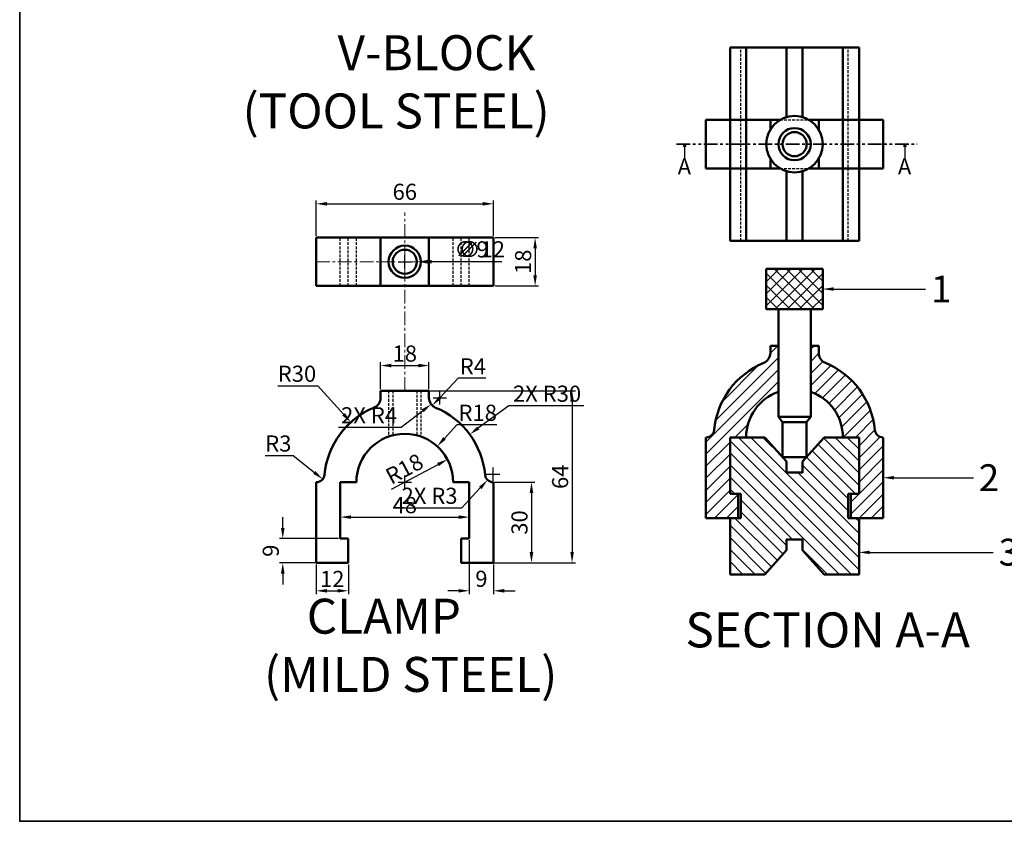
# Model space of a CAD drawing. Units: millimetres. Extents: x 0 to 624, y -214 to 340.
# Tile 1 of 3: x 0 to 366, y -214 to 84. Entities that reach past the tile are written whole.
import ezdxf
from ezdxf import colors
from ezdxf.entities.mleader import LeaderData, LeaderLine
from ezdxf.math import Vec2, Vec3

# ---------------------------------------------------------------- set-up
doc = ezdxf.new("R2010")
doc.units = ezdxf.units.MM
doc.header["$LTSCALE"] = 0.4
for name, pattern in [('CENTER', [50.8, 31.75, -6.35, 6.35, -6.35]), ('HIDDEN', [9.525, 6.35, -3.175]), ('PHANTOM', [63.5, 31.75, -6.35, 6.35, -6.35, 6.35, -6.35])]:
    doc.linetypes.add(name, pattern=pattern)
for name, color, linetype, lineweight in [('M-ANNO-SYMB', 6, 'Continuous', 25), ('M-CNTR', 1, 'CENTER', 18), ('M-DIMS', 2, 'Continuous', 25), ('M-HATC', 8, 'Continuous', 18), ('M-HIDN', 4, 'HIDDEN', 25), ('M-OUTL', 7, 'Continuous', 50), ('M-SECT', 6, 'PHANTOM', 35), ('M-TEXT', 3, 'Continuous', 25), ('M-TTLB', 7, 'Continuous', 35)]:
    doc.layers.add(name, color=color, linetype=linetype, lineweight=lineweight)
doc.styles.get("Standard").update_dxf_attribs({"font": 'arial.ttf'})
doc.dimstyles.new('ISO-25', dxfattribs={"dimtxt": 6, "dimasz": 4, "dimexe": 1.25, "dimexo": 0.625, "dimtad": 1, "dimtoh": 1, "dimtxsty": 'Standard', "dimcen": 2.5, "dimadec": 0, "dimazin": 0, "dimtfac": 1, "dimtofl": 0, "dimtmove": 0, "dimatfit": 3, "dimfxl": 1, "dimarcsym": 0})

# ---------------------------------------------------------------- blocks, each defined once
blk = doc.blocks.new('*D13')
at = {"layer": 'Defpoints', "color": 0, "ltscale": 0.4, "transparency": 16777216}
for p in [(176.26, 15.32), (110.26, 2.76), (176.26, 2.76)]:
    blk.add_point(p, dxfattribs=at)
at = {"layer": 'M-DIMS', "color": 0, "lineweight": -2, "ltscale": 0.4, "transparency": 16777216}
for p, q in [((110.26, 3.39), (110.26, 16.57)), ((114.26, 15.32), (172.26, 15.32)), ((176.26, 3.39), (176.26, 16.57))]:
    blk.add_line(p, q, dxfattribs=at)
at = {"layer": 'M-DIMS', "color": 0, "ltscale": 0.4, "transparency": 16777216}
for points in [[(114.26, 15.99), (114.26, 14.66), (110.26, 15.32)], [(172.26, 15.99), (172.26, 14.66), (176.26, 15.32)]]:
    blk.add_solid(points, dxfattribs=at)
at = {"layer": 'M-DIMS', "color": 0, "ltscale": 0.4, "transparency": 16777216, "insert": (143.26, 19.01), "char_height": 6, "attachment_point": 5}
blk.add_mtext('66', dxfattribs=at)
blk = doc.blocks.new('*D14')
at = {"layer": 'Defpoints', "color": 0, "ltscale": 0.4, "transparency": 16777216}
for p in [(176.26, 2.76), (176.26, -15.24), (191.74, -15.24)]:
    blk.add_point(p, dxfattribs=at)
at = {"layer": 'M-DIMS', "color": 0, "lineweight": -2, "ltscale": 0.4, "transparency": 16777216}
for p, q in [((176.88, 2.76), (192.99, 2.76)), ((191.74, -1.24), (191.74, -11.24)), ((176.88, -15.24), (192.99, -15.24))]:
    blk.add_line(p, q, dxfattribs=at)
at = {"layer": 'M-DIMS', "color": 0, "ltscale": 0.4, "transparency": 16777216}
for points in [[(191.07, -1.24), (192.4, -1.24), (191.74, 2.76)], [(191.07, -11.24), (192.4, -11.24), (191.74, -15.24)]]:
    blk.add_solid(points, dxfattribs=at)
at = {"layer": 'M-DIMS', "color": 0, "ltscale": 0.4, "transparency": 16777216, "insert": (188.05, -6.24), "char_height": 6, "attachment_point": 5, "rotation": 90}
blk.add_mtext('18', dxfattribs=at)
blk = doc.blocks.new('*D15')
at = {"layer": 'Defpoints', "color": 0, "ltscale": 0.4, "transparency": 16777216}
for p in [(119.26, -109.23), (97.87, -118.23), (119.26, -118.23)]:
    blk.add_point(p, dxfattribs=at)
at = {"layer": 'M-DIMS', "color": 0, "lineweight": -2, "ltscale": 0.4, "transparency": 16777216}
for p, q in [((97.87, -105.23), (97.87, -101.23)), ((118.63, -109.23), (96.62, -109.23)), ((118.63, -118.23), (96.62, -118.23)), ((97.87, -122.23), (97.87, -126.23))]:
    blk.add_line(p, q, dxfattribs=at)
at = {"layer": 'M-DIMS', "color": 0, "ltscale": 0.4, "transparency": 16777216}
for points in [[(97.2, -105.23), (98.53, -105.23), (97.87, -109.23)], [(97.2, -122.23), (98.53, -122.23), (97.87, -118.23)]]:
    blk.add_solid(points, dxfattribs=at)
at = {"layer": 'M-DIMS', "color": 0, "ltscale": 0.4, "transparency": 16777216, "insert": (94.18, -113.73), "char_height": 6, "attachment_point": 5, "rotation": 90}
blk.add_mtext('9', dxfattribs=at)
blk = doc.blocks.new('*D16')
at = {"layer": 'Defpoints', "color": 0, "ltscale": 0.4, "transparency": 16777216}
for p in [(119.26, -98.73), (167.26, -98.73), (167.26, -101.23)]:
    blk.add_point(p, dxfattribs=at)
at = {"layer": 'M-DIMS', "color": 0, "lineweight": -2, "ltscale": 0.4, "transparency": 16777216}
for p, q in [((119.26, -99.36), (119.26, -102.48)), ((123.26, -101.23), (163.26, -101.23)), ((167.26, -99.36), (167.26, -102.48))]:
    blk.add_line(p, q, dxfattribs=at)
at = {"layer": 'M-DIMS', "color": 0, "ltscale": 0.4, "transparency": 16777216}
for points in [[(123.26, -100.56), (123.26, -101.89), (119.26, -101.23)], [(163.26, -100.56), (163.26, -101.89), (167.26, -101.23)]]:
    blk.add_solid(points, dxfattribs=at)
at = {"layer": 'M-DIMS', "color": 0, "ltscale": 0.4, "transparency": 16777216, "insert": (143.26, -97.54), "char_height": 6, "attachment_point": 5}
blk.add_mtext('48', dxfattribs=at)
blk = doc.blocks.new('*D17')
at = {"layer": 'Defpoints', "color": 0, "ltscale": 0.4, "transparency": 16777216}
for p in [(176.12, -88.23), (176.26, -118.23), (190.39, -118.23)]:
    blk.add_point(p, dxfattribs=at)
at = {"layer": 'M-DIMS', "color": 0, "lineweight": -2, "ltscale": 0.4, "transparency": 16777216}
for p, q in [((176.75, -88.23), (191.64, -88.23)), ((190.39, -92.23), (190.39, -114.23)), ((176.88, -118.23), (191.64, -118.23))]:
    blk.add_line(p, q, dxfattribs=at)
at = {"layer": 'M-DIMS', "color": 0, "ltscale": 0.4, "transparency": 16777216}
for points in [[(189.73, -92.23), (191.06, -92.23), (190.39, -88.23)], [(189.73, -114.23), (191.06, -114.23), (190.39, -118.23)]]:
    blk.add_solid(points, dxfattribs=at)
at = {"layer": 'M-DIMS', "color": 0, "ltscale": 0.4, "transparency": 16777216, "insert": (186.7, -103.23), "char_height": 6, "attachment_point": 5, "rotation": 90}
blk.add_mtext('30', dxfattribs=at)
blk = doc.blocks.new('*D18')
at = {"layer": 'Defpoints', "color": 0, "ltscale": 0.4, "transparency": 16777216}
for p in [(143.26, -54.23), (164.26, -118.23), (205.5, -118.23)]:
    blk.add_point(p, dxfattribs=at)
at = {"layer": 'M-DIMS', "color": 0, "lineweight": -2, "ltscale": 0.4, "transparency": 16777216}
for p, q in [((143.88, -54.23), (206.75, -54.23)), ((205.5, -58.23), (205.5, -114.23)), ((164.88, -118.23), (206.75, -118.23))]:
    blk.add_line(p, q, dxfattribs=at)
at = {"layer": 'M-DIMS', "color": 0, "ltscale": 0.4, "transparency": 16777216}
for points in [[(204.84, -58.23), (206.17, -58.23), (205.5, -54.23)], [(204.84, -114.23), (206.17, -114.23), (205.5, -118.23)]]:
    blk.add_solid(points, dxfattribs=at)
at = {"layer": 'M-DIMS', "color": 0, "ltscale": 0.4, "transparency": 16777216, "insert": (201.82, -86.23), "char_height": 6, "attachment_point": 5, "rotation": 90}
blk.add_mtext('64', dxfattribs=at)
blk = doc.blocks.new('*D19')
at = {"layer": 'Defpoints', "color": 0, "ltscale": 0.4, "transparency": 16777216}
for p in [(152.26, -44.85), (134.26, -54.23), (152.26, -54.23)]:
    blk.add_point(p, dxfattribs=at)
at = {"layer": 'M-DIMS', "color": 0, "lineweight": -2, "ltscale": 0.4, "transparency": 16777216}
for p, q in [((134.26, -53.61), (134.26, -43.6)), ((152.26, -53.61), (152.26, -43.6)), ((138.26, -44.85), (148.26, -44.85))]:
    blk.add_line(p, q, dxfattribs=at)
at = {"layer": 'M-DIMS', "color": 0, "ltscale": 0.4, "transparency": 16777216}
for points in [[(138.26, -44.19), (138.26, -45.52), (134.26, -44.85)], [(148.26, -44.19), (148.26, -45.52), (152.26, -44.85)]]:
    blk.add_solid(points, dxfattribs=at)
at = {"layer": 'M-DIMS', "color": 0, "ltscale": 0.4, "transparency": 16777216, "insert": (143.26, -41.16), "char_height": 6, "attachment_point": 5}
blk.add_mtext('18', dxfattribs=at)
blk = doc.blocks.new('*D20')
at = {"layer": 'Defpoints', "color": 0, "ltscale": 0.4, "transparency": 16777216}
for p in [(159.15, -79.78), (143.26, -88.23)]:
    blk.add_point(p, dxfattribs=at)
at = {"layer": 'M-DIMS', "color": 0, "lineweight": -2, "ltscale": 0.4, "transparency": 16777216}
blk.add_line((138.32, -90.86), (155.62, -81.66), dxfattribs=at)
at = {"layer": 'M-DIMS', "color": 0, "ltscale": 0.4, "transparency": 16777216}
blk.add_solid([(155.3, -81.07), (155.93, -82.24), (159.15, -79.78)], dxfattribs=at)
at = {"layer": 'M-DIMS', "color": 0, "ltscale": 0.4, "transparency": 16777216, "insert": (143.47, -83.94), "char_height": 6, "attachment_point": 5, "rotation": 28.0255}
blk.add_mtext('R18', dxfattribs=at)
blk = doc.blocks.new('*D21')
at = {"layer": 'Defpoints', "color": 0, "ltscale": 0.4, "transparency": 16777216}
for p in [(123.18, -65.94), (143.26, -88.23)]:
    blk.add_point(p, dxfattribs=at)
at = {"layer": 'M-DIMS', "color": 0, "lineweight": -2, "ltscale": 0.4, "transparency": 16777216}
for p, q in [((96, -52.36), (110.94, -52.36)), ((110.94, -52.36), (120.5, -62.97)), ((143.26, -90.73), (143.26, -85.73)), ((140.76, -88.23), (145.76, -88.23))]:
    blk.add_line(p, q, dxfattribs=at)
at = {"layer": 'M-DIMS', "color": 0, "ltscale": 0.4, "transparency": 16777216}
blk.add_solid([(121, -62.53), (120.01, -63.42), (123.18, -65.94)], dxfattribs=at)
at = {"layer": 'M-DIMS', "color": 0, "ltscale": 0.4, "transparency": 16777216, "insert": (103.16, -48.67), "char_height": 6, "attachment_point": 5}
blk.add_mtext('R30', dxfattribs=at)
blk = doc.blocks.new('*D22')
at = {"layer": 'Defpoints', "color": 0, "ltscale": 0.4, "transparency": 16777216}
for p in [(110.39, -85.23), (112.74, -87.1)]:
    blk.add_point(p, dxfattribs=at)
at = {"layer": 'M-DIMS', "color": 0, "lineweight": -2, "ltscale": 0.4, "transparency": 16777216}
for p, q in [((91.38, -78.31), (101.68, -78.31)), ((101.68, -78.31), (109.61, -84.61))]:
    blk.add_line(p, q, dxfattribs=at)
at = {"layer": 'M-DIMS', "color": 0, "ltscale": 0.4, "transparency": 16777216}
blk.add_solid([(110.03, -84.09), (109.2, -85.13), (112.74, -87.1)], dxfattribs=at)
at = {"layer": 'M-DIMS', "color": 0, "ltscale": 0.4, "transparency": 16777216, "insert": (96.22, -74.62), "char_height": 6, "attachment_point": 5}
blk.add_mtext('R3', dxfattribs=at)
blk = doc.blocks.new('*D23')
at = {"layer": 'Defpoints', "color": 0, "ltscale": 0.4, "transparency": 16777216}
for p in [(156.26, -56.82), (153.51, -59.72)]:
    blk.add_point(p, dxfattribs=at)
at = {"layer": 'M-DIMS', "color": 0, "lineweight": -2, "ltscale": 0.4, "transparency": 16777216}
for p, q in [((163.14, -49.56), (156.26, -56.82)), ((173.41, -49.56), (163.14, -49.56))]:
    blk.add_line(p, q, dxfattribs=at)
at = {"layer": 'M-DIMS', "color": 0, "ltscale": 0.4, "transparency": 16777216}
blk.add_solid([(155.77, -56.36), (156.74, -57.28), (153.51, -59.72)], dxfattribs=at)
at = {"layer": 'M-DIMS', "color": 0, "ltscale": 0.4, "transparency": 16777216, "insert": (168.59, -45.93), "char_height": 6, "attachment_point": 5}
blk.add_mtext('R4', dxfattribs=at)
blk = doc.blocks.new('SECTION-ARROW')
at = {"ltscale": 0.4}
for p, q in [((0.5, 5.29), (0, 4.42)), ((1, 4.42), (0, 4.42)), ((0.5, 5.29), (0.5, 0)), ((0.5, 5.29), (1, 4.42))]:
    blk.add_line(p, q, dxfattribs=at)
blk = doc.blocks.new('*D38')
at = {"layer": 'Defpoints', "color": 0, "ltscale": 0.4, "transparency": 16777216}
for p in [(110.26, -118.23), (122.26, -118.23), (122.26, -128.63)]:
    blk.add_point(p, dxfattribs=at)
at = {"layer": 'M-DIMS', "color": 0, "lineweight": -2, "ltscale": 0.4, "transparency": 16777216}
for p, q in [((110.26, -118.86), (110.26, -129.88)), ((122.26, -118.86), (122.26, -129.88)), ((114.26, -128.63), (118.26, -128.63))]:
    blk.add_line(p, q, dxfattribs=at)
at = {"layer": 'M-DIMS', "color": 0, "ltscale": 0.4, "transparency": 16777216}
for points in [[(114.26, -127.97), (114.26, -129.3), (110.26, -128.63)], [(118.26, -127.97), (118.26, -129.3), (122.26, -128.63)]]:
    blk.add_solid(points, dxfattribs=at)
at = {"layer": 'M-DIMS', "color": 0, "ltscale": 0.4, "transparency": 16777216, "insert": (116.26, -125), "char_height": 6, "attachment_point": 5}
blk.add_mtext('12', dxfattribs=at)
blk = doc.blocks.new('*D39')
at = {"layer": 'Defpoints', "color": 0, "ltscale": 0.4, "transparency": 16777216}
for p in [(167.26, -109.23), (176.26, -118.23), (176.26, -128.63)]:
    blk.add_point(p, dxfattribs=at)
at = {"layer": 'M-DIMS', "color": 0, "lineweight": -2, "ltscale": 0.4, "transparency": 16777216}
for p, q in [((167.26, -109.86), (167.26, -129.88)), ((176.26, -118.86), (176.26, -129.88)), ((163.26, -128.63), (159.26, -128.63)), ((180.26, -128.63), (184.26, -128.63))]:
    blk.add_line(p, q, dxfattribs=at)
at = {"layer": 'M-DIMS', "color": 0, "ltscale": 0.4, "transparency": 16777216}
for points in [[(163.26, -127.97), (163.26, -129.3), (167.26, -128.63)], [(180.26, -127.97), (180.26, -129.3), (176.26, -128.63)]]:
    blk.add_solid(points, dxfattribs=at)
at = {"layer": 'M-DIMS', "color": 0, "ltscale": 0.4, "transparency": 16777216, "insert": (171.76, -124.95), "char_height": 6, "attachment_point": 5}
blk.add_mtext('9', dxfattribs=at)
blk = doc.blocks.new('*D41')
at = {"layer": 'Defpoints', "color": 0, "ltscale": 0.4, "transparency": 16777216}
for p in [(167.42, -70.44), (143.26, -88.23)]:
    blk.add_point(p, dxfattribs=at)
at = {"layer": 'M-DIMS', "color": 0, "lineweight": -2, "ltscale": 0.4, "transparency": 16777216}
for p, q in [((181.91, -59.77), (170.64, -68.07)), ((209.85, -59.77), (181.91, -59.77)), ((143.26, -90.73), (143.26, -85.73)), ((140.76, -88.23), (145.76, -88.23))]:
    blk.add_line(p, q, dxfattribs=at)
at = {"layer": 'M-DIMS', "color": 0, "ltscale": 0.4, "transparency": 16777216}
blk.add_solid([(170.24, -67.54), (171.03, -68.61), (167.42, -70.44)], dxfattribs=at)
at = {"layer": 'M-DIMS', "color": 0, "ltscale": 0.4, "transparency": 16777216, "insert": (196.19, -56.08), "char_height": 6, "attachment_point": 5}
blk.add_mtext('2X R30', dxfattribs=at)
blk = doc.blocks.new('*D42')
at = {"layer": 'Defpoints', "color": 0, "ltscale": 0.4, "transparency": 16777216}
for p in [(155.34, -74.89), (143.26, -88.23)]:
    blk.add_point(p, dxfattribs=at)
at = {"layer": 'M-DIMS', "color": 0, "lineweight": -2, "ltscale": 0.4, "transparency": 16777216}
for p, q in [((162.59, -66.88), (158.02, -71.92)), ((177.56, -66.88), (162.59, -66.88)), ((143.26, -90.73), (143.26, -85.73)), ((140.76, -88.23), (145.76, -88.23))]:
    blk.add_line(p, q, dxfattribs=at)
at = {"layer": 'M-DIMS', "color": 0, "ltscale": 0.4, "transparency": 16777216}
blk.add_solid([(157.53, -71.48), (158.52, -72.37), (155.34, -74.89)], dxfattribs=at)
at = {"layer": 'M-DIMS', "color": 0, "ltscale": 0.4, "transparency": 16777216, "insert": (170.39, -63.19), "char_height": 6, "attachment_point": 5}
blk.add_mtext('R18', dxfattribs=at)
blk = doc.blocks.new('*D43')
at = {"layer": 'Defpoints', "color": 0, "ltscale": 0.4, "transparency": 16777216}
for p in [(156.26, -56.82), (153.08, -59.24)]:
    blk.add_point(p, dxfattribs=at)
at = {"layer": 'M-DIMS', "color": 0, "lineweight": -2, "ltscale": 0.4, "transparency": 16777216}
for p, q in [((156.26, -59.32), (156.26, -54.32)), ((153.76, -56.82), (158.76, -56.82)), ((141.93, -67.76), (149.9, -61.67)), ((118.66, -67.76), (141.93, -67.76))]:
    blk.add_line(p, q, dxfattribs=at)
at = {"layer": 'M-DIMS', "color": 0, "ltscale": 0.4, "transparency": 16777216}
blk.add_solid([(149.5, -61.14), (150.3, -62.2), (153.08, -59.24)], dxfattribs=at)
at = {"layer": 'M-DIMS', "color": 0, "ltscale": 0.4, "transparency": 16777216, "insert": (129.98, -64.12), "char_height": 6, "attachment_point": 5}
blk.add_mtext('2X R4', dxfattribs=at)
blk = doc.blocks.new('*D44')
at = {"layer": 'Defpoints', "color": 0, "ltscale": 0.4, "transparency": 16777216}
for p in [(174.07, -87.43), (176.12, -85.23)]:
    blk.add_point(p, dxfattribs=at)
at = {"layer": 'M-DIMS', "color": 0, "lineweight": -2, "ltscale": 0.4, "transparency": 16777216}
for p, q in [((176.12, -87.73), (176.12, -82.73)), ((173.62, -85.23), (178.62, -85.23)), ((164.43, -97.76), (171.35, -90.35)), ((141.14, -97.76), (164.43, -97.76))]:
    blk.add_line(p, q, dxfattribs=at)
at = {"layer": 'M-DIMS', "color": 0, "ltscale": 0.4, "transparency": 16777216}
blk.add_solid([(170.86, -89.9), (171.83, -90.81), (174.07, -87.43)], dxfattribs=at)
at = {"layer": 'M-DIMS', "color": 0, "ltscale": 0.4, "transparency": 16777216, "insert": (152.47, -94.07), "char_height": 6, "attachment_point": 5}
blk.add_mtext('2X R3', dxfattribs=at)
blk = doc.blocks.new('*D45')
at = {"layer": 'Defpoints', "color": 0, "ltscale": 0.4, "transparency": 16777216}
for p in [(137.26, -6.24), (149.26, -6.24)]:
    blk.add_point(p, dxfattribs=at)
at = {"layer": 'M-DIMS', "color": 0, "lineweight": -2, "ltscale": 0.4, "transparency": 16777216}
for p, q in [((140.76, -6.24), (145.76, -6.24)), ((143.26, -8.74), (143.26, -3.74)), ((163.72, -6.24), (153.26, -6.24)), ((179.41, -6.24), (163.72, -6.24))]:
    blk.add_line(p, q, dxfattribs=at)
at = {"layer": 'M-DIMS', "color": 0, "ltscale": 0.4, "transparency": 16777216}
blk.add_solid([(153.26, -5.57), (153.26, -6.91), (149.26, -6.24)], dxfattribs=at)
at = {"layer": 'M-DIMS', "color": 0, "ltscale": 0.4, "transparency": 16777216, "insert": (171.88, -2.39), "char_height": 6, "attachment_point": 5}
blk.add_mtext('∅12', dxfattribs=at)
blk = doc.blocks.new('*D46')
at = {"layer": 'Defpoints', "color": 0, "ltscale": 0.4, "transparency": 16777216}
for p in [(138.76, -6.24), (147.76, -6.24)]:
    blk.add_point(p, dxfattribs=at)
at = {"layer": 'M-DIMS', "color": 0, "lineweight": -2, "ltscale": 0.4, "transparency": 16777216}
for p, q in [((140.76, -6.24), (145.76, -6.24)), ((143.26, -8.74), (143.26, -3.74)), ((162.22, -6.24), (151.76, -6.24)), ((173.32, -6.24), (162.22, -6.24))]:
    blk.add_line(p, q, dxfattribs=at)
at = {"layer": 'M-DIMS', "color": 0, "ltscale": 0.4, "transparency": 16777216}
blk.add_solid([(151.76, -5.57), (151.76, -6.91), (147.76, -6.24)], dxfattribs=at)
at = {"layer": 'M-DIMS', "color": 0, "ltscale": 0.4, "transparency": 16777216, "insert": (168.08, -2.39), "char_height": 6, "attachment_point": 5}
blk.add_mtext('∅9', dxfattribs=at)

msp = doc.modelspace()

# ---------------------------------------------------------------- hatches: boundary and pattern name
at = {"layer": 'M-HATC', "ltscale": 0.4}
h = msp.add_hatch(dxfattribs=at)
h.set_pattern_fill('ANSI37', color=256)
h.set_pattern_definition([(45, (-210.0675, -178.2087), (-2.245064, 2.245064), []), (135, (-210.0675, -178.2087), (-2.245064, -2.245064), [])])
h.paths.add_polyline_path([(277.758, -23.89), (298.758, -23.89), (298.758, -8.89), (277.758, -8.89)])
h = msp.add_hatch(dxfattribs=at)
h.set_pattern_fill('ANSI31', color=256)
h.set_pattern_definition([(45, (412.649, -284.1122), (-2.245064, 2.245064), [])])
h.paths.add_polyline_path([(306.25, -71.568), (312.25, -71.568), (312.25, -92.568), (309.25, -92.568), (309.25, -101.568), (312.25, -101.568), (321.25, -101.568), (321.25, -71.568), (321.113, -71.568, -0.3877946), (318.126, -68.841, 0.2787563), (299.72, -43.847, -0.3034443), (297.25, -40.151), (297.25, -37.568), (294.258, -37.568), (294.258, -54.6, -0.3176981)])
h.paths.add_polyline_path([(282.258, -54.594), (282.258, -37.568), (279.25, -37.568), (279.25, -40.151, -0.3034443), (276.779, -43.847, 0.2787563), (258.374, -68.841, -0.3877946), (255.386, -71.568), (255.25, -71.568), (255.25, -101.568), (264.25, -101.568), (267.25, -101.568), (267.25, -92.568), (264.25, -92.568), (264.25, -71.568), (270.25, -71.568, -0.3179764)])
h = msp.add_hatch(dxfattribs=at)
h.set_pattern_fill('ANSI31', color=256, angle=90)
h.set_pattern_definition([(135, (412.649, -284.1122), (-2.245064, -2.245064), [])])
h.paths.add_polyline_path([(308.25, -92.568), (312.25, -92.568), (312.25, -71.568), (306.25, -71.568), (299.25, -71.568), (292.758, -78.871), (292.758, -78.89), (292.741, -78.89), (291.25, -80.568), (291.25, -84.568), (288.25, -84.568), (285.25, -84.568), (285.25, -80.568), (277.25, -71.568), (264.25, -71.568), (264.25, -92.568), (267.25, -92.568), (268.25, -92.568), (268.25, -101.568), (264.25, -101.568), (264.25, -122.568), (277.25, -122.568), (285.25, -113.568), (285.25, -109.568), (288.25, -109.568), (291.25, -109.568), (291.25, -113.568), (299.25, -122.568), (312.25, -122.568), (312.25, -101.568), (309.25, -101.568), (308.25, -101.568)])

# ---------------------------------------------------------------- linework, layer by layer
at = {"layer": 'M-CNTR', "ltscale": 0.4}
for p, q in [((143.258, -54.234), (143.258, 12.04)), ((110.258, -6.239), (176.258, -6.239))]:
    msp.add_line(p, q, dxfattribs=at)
at = {"layer": 'M-HIDN', "ltscale": 0.4}
for p, q in [((268.258, 1.51), (268.258, 73.51)), ((308.258, 1.51), (308.258, 73.51)), ((264.258, 28.51), (264.258, 46.51)), ((270.258, 28.51), (270.258, 46.51)), ((282.85, 46.51), (293.667, 46.51)), ((306.258, 28.51), (306.258, 46.51)), ((312.258, 28.51), (312.258, 46.51)), ((282.85, 28.51), (293.667, 28.51)), ((119.258, -15.239), (119.258, 2.761)), ((122.258, -15.239), (122.258, 2.761)), ((125.258, -15.239), (125.258, 2.761)), ((161.258, -15.239), (161.258, 2.761)), ((164.258, -15.239), (164.258, 2.761)), ((167.258, -15.239), (167.258, 2.761)), ((137.258, -54.234), (137.258, -71.263)), ((138.758, -54.234), (138.758, -70.805)), ((147.758, -54.234), (147.758, -70.805)), ((149.258, -54.234), (149.258, -71.263))]:
    msp.add_line(p, q, dxfattribs=at)
at = {"layer": 'M-OUTL', "ltscale": 0.4}
for p, q in [((312.258, 73.51), (264.258, 73.51)), ((264.258, 73.51), (264.258, 1.51)), ((270.258, 73.51), (270.258, 1.51)), ((285.258, 47.573), (285.258, 73.51)), ((291.258, 47.573), (291.258, 73.51)), ((306.258, 1.51), (306.258, 73.51)), ((312.258, 1.51), (312.258, 73.51)), ((255.258, 46.51), (255.258, 28.51)), ((282.85, 46.51), (255.258, 46.51)), ((279.258, 46.51), (279.258, 42.919)), ((321.258, 46.51), (293.667, 46.51)), ((297.258, 46.51), (297.258, 42.919)), ((321.258, 28.51), (321.258, 46.51)), ((279.258, 32.102), (279.258, 28.51)), ((297.258, 32.102), (297.258, 28.51)), ((255.258, 28.51), (282.85, 28.51)), ((285.258, 1.51), (285.258, 27.448)), ((291.258, 1.51), (291.258, 27.448)), ((293.667, 28.51), (321.258, 28.51)), ((176.258, 2.761), (110.258, 2.761)), ((110.258, 2.761), (110.258, -15.239)), ((134.258, 2.761), (134.258, -15.239)), ((152.258, 2.761), (152.258, -15.239)), ((176.258, -15.239), (176.258, 2.761)), ((264.258, 1.51), (288.258, 1.51)), ((288.258, 1.51), (312.258, 1.51)), ((298.758, -8.89), (277.758, -8.89)), ((277.758, -8.89), (277.758, -23.89)), ((298.758, -23.89), (298.758, -8.89)), ((110.258, -15.239), (143.258, -15.239)), ((143.258, -15.239), (176.258, -15.239)), ((277.758, -23.89), (298.758, -23.89)), ((282.258, -23.89), (282.258, -63.89)), ((294.258, -63.89), (294.258, -23.89)), ((279.25, -37.568), (282.258, -37.568)), ((279.25, -37.568), (279.25, -40.151)), ((294.258, -37.568), (297.25, -37.568)), ((297.25, -37.568), (297.25, -40.151)), ((134.258, -54.234), (152.258, -54.234)), ((134.258, -54.234), (134.258, -56.817)), ((152.258, -54.234), (152.258, -56.817)), ((292.758, -63.89), (282.258, -63.89)), ((282.258, -63.89), (283.758, -65.89)), ((292.758, -65.89), (283.758, -65.89)), ((283.758, -78.89), (283.758, -65.89)), ((294.258, -63.89), (292.758, -63.89)), ((294.258, -63.89), (292.758, -65.89)), ((292.758, -78.89), (292.758, -65.89)), ((255.25, -71.568), (255.25, -101.568)), ((255.386, -71.568), (255.25, -71.568)), ((264.25, -71.568), (270.25, -71.568)), ((264.25, -71.568), (264.25, -92.568)), ((306.25, -71.568), (312.25, -71.568)), ((312.25, -71.568), (312.25, -92.568)), ((321.113, -71.568), (321.25, -71.568)), ((321.25, -71.568), (321.25, -101.568)), ((288.258, -78.89), (283.758, -78.89)), ((288.258, -78.89), (292.758, -78.89)), ((110.258, -88.234), (110.258, -118.234)), ((110.395, -88.234), (110.258, -88.234)), ((119.258, -88.234), (125.258, -88.234)), ((119.258, -88.234), (119.258, -109.234)), ((161.258, -88.234), (167.258, -88.234)), ((167.258, -88.234), (167.258, -109.234)), ((176.122, -88.234), (176.258, -88.234)), ((176.258, -88.234), (176.258, -118.234)), ((264.25, -92.568), (267.25, -92.568)), ((267.25, -92.568), (267.25, -101.568)), ((312.25, -92.568), (309.25, -92.568)), ((309.25, -92.568), (309.25, -101.568)), ((255.25, -101.568), (264.25, -101.568)), ((267.25, -101.568), (264.25, -101.568)), ((309.25, -101.568), (312.25, -101.568)), ((312.25, -101.568), (321.25, -101.568)), ((119.258, -109.234), (122.258, -109.234)), ((122.258, -109.234), (122.258, -118.234)), ((167.258, -109.234), (164.258, -109.234)), ((164.258, -109.234), (164.258, -118.234)), ((110.258, -118.234), (119.258, -118.234)), ((122.258, -118.234), (119.258, -118.234)), ((164.258, -118.234), (167.258, -118.234)), ((167.258, -118.234), (176.258, -118.234))]:
    msp.add_line(p, q, dxfattribs=at)
at = {"layer": 'M-OUTL'}
for p, q in [((264.25, -71.568), (264.25, -92.568)), ((277.25, -71.568), (264.25, -71.568)), ((312.25, -71.568), (299.25, -71.568)), ((312.25, -92.568), (312.25, -71.568)), ((264.25, -92.568), (268.25, -92.568)), ((268.25, -92.568), (268.25, -101.568)), ((308.25, -101.568), (308.25, -92.568)), ((308.25, -92.568), (312.25, -92.568)), ((268.25, -101.568), (264.25, -101.568)), ((264.25, -101.568), (264.25, -122.568)), ((312.25, -101.568), (308.25, -101.568)), ((312.25, -122.568), (312.25, -101.568)), ((264.25, -109.568), (264.25, -122.568)), ((264.25, -122.568), (277.25, -122.568)), ((299.25, -122.568), (312.25, -122.568))]:
    msp.add_line(p, q, dxfattribs=at)
for points in [[(277.25, -71.568), (285.25, -80.568), (285.25, -84.568), (288.25, -84.568), (291.25, -84.568), (291.25, -80.568), (299.25, -71.568)], [(277.25, -122.568), (285.25, -113.568), (285.25, -109.568), (288.25, -109.568), (291.25, -109.568), (291.25, -113.568), (299.25, -122.568)]]:
    msp.add_lwpolyline(points, dxfattribs=at)
at = {"layer": 'M-OUTL', "ltscale": 0.4}
for centre, radius in [((288.258, 37.51), 10.5), ((288.258, 37.51), 6), ((288.258, 37.51), 4.5), ((143.258, -6.239), 6), ((143.258, -6.239), 4.5)]:
    msp.add_circle(centre, radius, dxfattribs=at)
for centre, radius, start, end in [((275.25, -40.151), 4, 292.47951, 0), ((301.25, -40.151), 4, 180, 247.52049), ((288.25, -71.568), 30, 112.47951, 174.78409), ((288.25, -71.568), 30, 5.21591, 67.52049), ((288.25, -71.568), 18, 109.44225, 180), ((288.25, -71.568), 18, 0, 70.49981), ((130.258, -56.817), 4, 292.47951, 0), ((156.258, -56.817), 4, 180, 247.52049), ((143.258, -88.234), 30, 112.47951, 174.78409), ((143.258, -88.234), 30, 5.21591, 67.52049), ((255.386, -68.568), 3, 270, 354.78409), ((321.113, -68.568), 3, 185.21591, 270), ((143.258, -88.234), 18, 0, 180), ((110.395, -85.234), 3, 270, 354.78409), ((176.122, -85.234), 3, 185.21591, 270)]:
    msp.add_arc(centre, radius, start, end, dxfattribs=at)
at = {"layer": 'M-SECT', "ltscale": 0.4}
msp.add_line((244.354, 37.51), (333.877, 37.51), dxfattribs=at)
at = {"layer": 'M-TTLB', "ltscale": 0.4}
msp.add_lwpolyline([(0, 340.107), (623.623, 340.107), (623.623, -214.379), (0, -214.379)], close=True, dxfattribs=at)

# ---------------------------------------------------------------- block references
at = {"layer": 'M-ANNO-SYMB'}
for p in [(246.833, 32.22), (328.744, 32.22)]:
    msp.add_blockref('SECTION-ARROW', p, dxfattribs=at)

# ---------------------------------------------------------------- texts
at = {"layer": 'M-TEXT', "ltscale": 0.4, "attachment_point": 1}
for s, width, insert, char_height in [('\\pxqc;V-BLOCK\\P\\pq*;  (TOOL STEEL)', 160.14315, (74.965, 78.033), 13), ('A', 4.82335, (244.793, 32.242), 6), ('A', 4.82335, (326.704, 32.242), 6), ('        CLAMP\\P    (MILD STEEL)', 160.14315, (75.008, -131.574), 13), ('\\pxqc;SECTION A-A', 160.14315, (220.499, -136.678), 13)]:
    msp.add_mtext_dynamic_manual_height_columns(s, width=width, gutter_width=12.5, heights=[0], dxfattribs=dict(at, insert=insert, char_height=char_height))

# ---------------------------------------------------------------- dimensions: what is measured, and where the dimension line sits
at = {"layer": 'M-DIMS', "ltscale": 0.4}
for base, p1, p2, override, picture, middle in [((176.258, 15.323), (110.258, 2.761), (176.258, 2.761), {"dimclrd": 0, "dimclre": 0, "dimclrt": 0}, '*D13', (143.258, 19.012)), ((152.258, -44.852), (134.258, -54.234), (152.258, -54.234), {"dimclrd": 0, "dimclre": 0, "dimclrt": 0}, '*D19', (143.258, -41.164)), ((167.258, -101.227), (119.258, -98.734), (167.258, -98.734), {"dimclrd": 0, "dimclre": 0, "dimclrt": 0}, '*D16', (143.258, -97.538)), ((176.258, -128.634), (167.258, -109.234), (176.258, -118.234), {"dimdec": 0, "dimlfac": 1, "dimrnd": 0, "dimzin": 0, "dimdsep": 46, "dimlunit": 2}, '*D39', (171.758, -124.945)), ((122.258, -128.634), (110.258, -118.234), (122.258, -118.234), {"dimdec": 0, "dimlfac": 1, "dimrnd": 0, "dimzin": 0, "dimdsep": 46, "dimlunit": 2}, '*D38', (116.258, -124.997))]:
    dim = msp.add_linear_dim(base=base, p1=p1, p2=p2, dimstyle='ISO-25', override=override, dxfattribs=at)
    dim.commit()
    dim.dimension.update_dxf_attribs({"geometry": picture, "text_midpoint": middle})
for p1, p2, picture, middle in [((137.258, -6.239), (149.258, -6.24), '*D45', (163.721, -6.241)), ((138.758, -6.239), (147.758, -6.24), '*D46', (162.221, -6.242))]:
    dim = msp.add_diameter_dim_2p(p1=p1, p2=p2, dimstyle='ISO-25', override={"dimdec": 0, "dimlfac": 1, "dimrnd": 0, "dimzin": 0, "dimdsep": 46, "dimlunit": 2}, dxfattribs=at)
    dim.commit()
    dim.dimension.update_dxf_attribs({"geometry": picture, "text_midpoint": middle, "dimtype": 163})
for base, p1, p2, picture, middle in [((191.738, -15.239), (176.258, 2.761), (176.258, -15.239), '*D14', (188.05, -6.239)), ((205.504, -118.234), (143.258, -54.234), (164.258, -118.234), '*D18', (201.815, -86.234)), ((190.392, -118.234), (176.122, -88.234), (176.258, -118.234), '*D17', (186.701, -103.234)), ((97.866, -118.234), (119.258, -109.234), (119.258, -118.234), '*D15', (94.177, -113.734))]:
    dim = msp.add_linear_dim(base=base, p1=p1, p2=p2, angle=90, dimstyle='ISO-25', override={"dimclrd": 0, "dimclre": 0, "dimclrt": 0}, dxfattribs=at)
    dim.commit()
    dim.dimension.update_dxf_attribs({"geometry": picture, "text_midpoint": middle})
for center, mpoint, override, picture, middle in [((156.258, -56.817), (153.507, -59.72), {"dimclrd": 0, "dimclre": 0, "dimclrt": 0}, '*D23', (168.588, -49.559)), ((143.258, -88.234), (123.179, -65.944), {"dimclrd": 0, "dimclre": 0, "dimclrt": 0}, '*D21', (103.156, -52.358)), ((143.258, -88.234), (155.338, -74.889), {"dimdec": 0, "dimlfac": 1, "dimrnd": 0, "dimzin": 0, "dimdsep": 46, "dimlunit": 2}, '*D42', (170.386, -66.883)), ((110.395, -85.234), (112.744, -87.1), {"dimclrd": 0, "dimclre": 0, "dimclrt": 0}, '*D22', (96.217, -78.31)), ((143.258, -88.234), (159.148, -79.776), {"dimclrd": 0, "dimclre": 0, "dimclrt": 0}, '*D20', (145.201, -87.2))]:
    dim = msp.add_radius_dim(center=center, mpoint=mpoint, dimstyle='ISO-25', override=override, dxfattribs=at)
    dim.commit()
    dim.dimension.update_dxf_attribs({"geometry": picture, "text_midpoint": middle, "dimtype": 164})
dim = msp.add_radius_dim(center=(143.258, -88.234), mpoint=(167.415, -70.445), text='2X <>', dimstyle='ISO-25', override={"dimdec": 0, "dimlfac": 1, "dimrnd": 0, "dimzin": 0, "dimdsep": 46, "dimlunit": 2}, dxfattribs=at)
dim.commit()
dim.dimension.update_dxf_attribs({"geometry": '*D41', "text_midpoint": (196.19, -59.772), "dimtype": 164})
for center, mpoint, picture, middle in [((156.258, -56.817), (153.079, -59.245), '*D43', (129.982, -64.12)), ((176.122, -85.234), (174.075, -87.427), '*D44', (152.473, -94.067))]:
    dim = msp.add_radius_dim(center=center, mpoint=mpoint, text='2X <>', dimstyle='ISO-25', override={"dimdec": 0, "dimlfac": 1, "dimrnd": 0, "dimzin": 0, "dimdsep": 46, "dimlunit": 2}, dxfattribs=at)
    dim.commit()
    dim.dimension.update_dxf_attribs({"geometry": picture, "text_midpoint": middle})

# ---------------------------------------------------------------- leaders
at = {"layer": 'M-TEXT', "ltscale": 0.4}
ml = msp.add_multileader_mtext('Standard', dxfattribs=at)
ml.set_content('1', color=256)
ml.set_leader_properties()
ml.build(insert=Vec2(0, 0))
ctx = ml.context
ctx.base_point, ctx.char_height, ctx.plane_origin = Vec3(336.999, -16.39), 10, Vec3(298.758, -16.39)
notes = []
notes.append((ctx, [(0, (1, 1, 0), (328.999, -16.39), (1, 0), 8, [(0, [(298.758, -16.39)], 0, [])])]))
ctx.mtext.insert, ctx.mtext.flow_direction = Vec3(338.999, -11.39), 5
ml = msp.add_multileader_mtext('Standard', dxfattribs=at)
ml.set_content('2', color=256)
ml.set_leader_properties()
ml.build(insert=Vec2(0, 0))
ctx = ml.context
ctx.base_point, ctx.char_height, ctx.plane_origin = Vec3(354.793, -86.568), 10, Vec3(321.25, -86.568)
notes.append((ctx, [(0, (1, 1, 0), (346.793, -86.568), (1, 0), 8, [(0, [(321.25, -86.568)], 0, [])])]))
ctx.mtext.insert, ctx.mtext.flow_direction = Vec3(356.793, -81.568), 5
ml = msp.add_multileader_mtext('Standard', dxfattribs=at)
ml.set_content('3', color=256)
ml.set_leader_properties()
ml.build(insert=Vec2(0, 0))
ctx = ml.context
ctx.base_point, ctx.char_height, ctx.plane_origin = Vec3(362.19, -114.345), 10, Vec3(312.25, -114.345)
notes.append((ctx, [(0, (1, 1, 0), (354.19, -114.345), (1, 0), 8, [(0, [(312.25, -114.345)], 0, [])])]))
ctx.mtext.insert, ctx.mtext.flow_direction = Vec3(364.19, -109.256), 5
for ctx, leaders in notes:
    for number, flags, end, landing, length, lines in leaders:
        leader = LeaderData()
        leader.index, (leader.has_last_leader_line, leader.has_dogleg_vector, leader.attachment_direction) = number, flags
        leader.last_leader_point, leader.dogleg_vector, leader.dogleg_length = Vec3(end), Vec3(landing), length
        for number, points, colour, breaks in lines:
            line = LeaderLine()
            line.index, line.vertices, line.color, line.breaks = number, Vec3.list(points), colors.encode_raw_color(colour), breaks
            leader.lines.append(line)
        ctx.leaders.append(leader)

doc.saveas('drawing.dxf')
